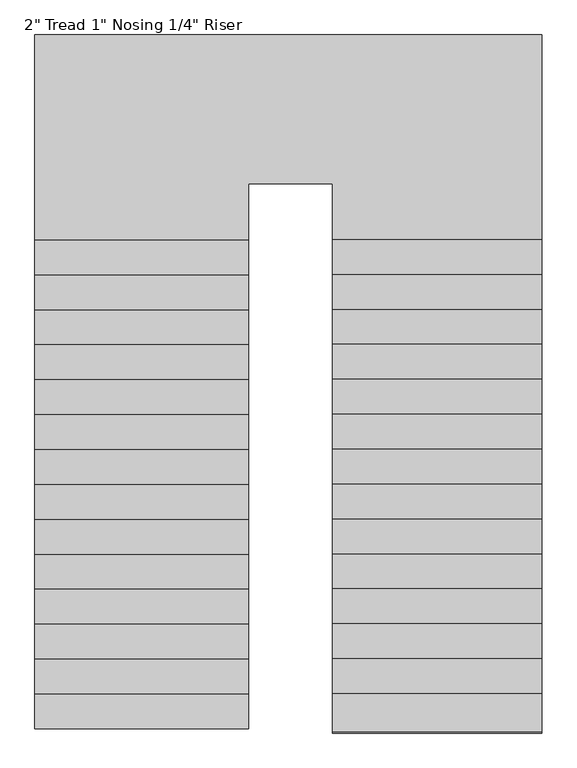
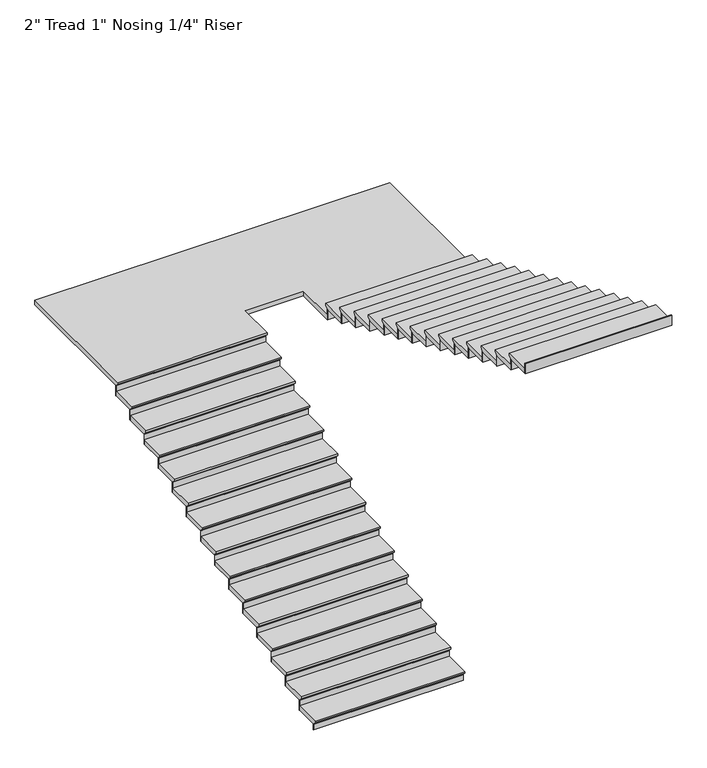
"""IFC4 building model written with IfcOpenShell, lengths in millimetres: stair flight geometry."""

from ifc_helpers import new_model, si_unit, origin, place, context, project, spatial, faceted_brep, source, transform, mapped, element, save


def stair_flight_b71c2a3e(model_context):
    return source(origin(), model_context, "Body", "Brep", [
        faceted_brep([(-5999.9290366, -6973.0610642, -212.09), (-5999.9290366, -6973.0610642, -193.04), (-7554.4415084, -6973.0610642, -193.04), (-7554.4415084, -6973.0610642, -212.09), (-5999.9290366, -6947.6610642, -237.49), (-7554.4415084, -6947.6610642, -237.49), (-5999.9290366, -6693.6610642, -193.04), (-7554.4415084, -6693.6610642, -193.04), (-7554.4415084, -6947.6610642, -243.84), (-7554.4415084, -6693.6610642, -243.84), (-5999.9290366, -6693.6610642, -243.84), (-5999.9290366, -6947.6610642, -243.84)], [[[0, 1, 2, 3]], [[4, 0, 3, 5]], [[2, 1, 6, 7]], [[8, 9, 10, 11]], [[2, 7, 9, 8, 5, 3]], [[8, 11, 4, 5]], [[6, 1, 0, 4, 11, 10]], [[7, 6, 10, 9]]]),
        faceted_brep([(-5999.9290366, -6947.6610642, -243.84), (-5999.9290366, -6947.6610642, -304.8), (-5999.9290366, -6941.3110642, -304.8), (-5999.9290366, -6941.3110642, -243.84), (-7554.4415084, -6947.6610642, -243.84), (-7554.4415084, -6941.3110642, -243.84), (-7554.4415084, -6941.3110642, -304.8), (-7554.4415084, -6947.6610642, -304.8)], [[[0, 1, 2, 3]], [[4, 5, 6, 7]], [[1, 0, 4, 7]], [[2, 1, 7, 6]], [[3, 2, 6, 5]], [[0, 3, 5, 4]]]),
        faceted_brep([(-5999.9290366, -6693.6610642, -132.08), (-5999.9290366, -6693.6610642, -243.84), (-5999.9290366, -6687.3110642, -243.84), (-5999.9290366, -6687.3110642, -132.08), (-7554.4415084, -6693.6610642, -132.08), (-7554.4415084, -6687.3110642, -132.08), (-7554.4415084, -6687.3110642, -243.84), (-7554.4415084, -6693.6610642, -243.84)], [[[0, 1, 2, 3]], [[4, 5, 6, 7]], [[1, 0, 4, 7]], [[2, 1, 7, 6]], [[3, 2, 6, 5]], [[0, 3, 5, 4]]]),
        faceted_brep([(-7554.4415084, -6719.0610642, -81.28), (-5999.9290366, -6719.0610642, -81.28), (-5999.9290366, -6439.6610642, -81.28), (-7554.4415084, -6439.6610642, -81.28), (-7554.4415084, -6693.6610642, -132.08), (-7554.4415084, -6439.6610642, -132.08), (-5999.9290366, -6439.6610642, -132.08), (-5999.9290366, -6693.6610642, -132.08), (-7554.4415084, -6693.6610642, -125.73), (-7554.4415084, -6719.0610642, -100.33), (-5999.9290366, -6693.6610642, -125.73), (-5999.9290366, -6719.0610642, -100.33)], [[[0, 1, 2, 3]], [[4, 5, 6, 7]], [[0, 3, 5, 4, 8, 9]], [[4, 7, 10, 8]], [[2, 1, 11, 10, 7, 6]], [[3, 2, 6, 5]], [[11, 1, 0, 9]], [[10, 11, 9, 8]]]),
        faceted_brep([(-5999.9290366, -6439.6610642, -20.32), (-5999.9290366, -6439.6610642, -132.08), (-5999.9290366, -6433.3110642, -132.08), (-5999.9290366, -6433.3110642, -20.32), (-7554.4415084, -6439.6610642, -20.32), (-7554.4415084, -6433.3110642, -20.32), (-7554.4415084, -6433.3110642, -132.08), (-7554.4415084, -6439.6610642, -132.08)], [[[0, 1, 2, 3]], [[4, 5, 6, 7]], [[1, 0, 4, 7]], [[2, 1, 7, 6]], [[3, 2, 6, 5]], [[0, 3, 5, 4]]]),
        faceted_brep([(-7554.4415084, -6465.0610642, 30.48), (-5999.9290366, -6465.0610642, 30.48), (-5999.9290366, -6185.6610642, 30.48), (-7554.4415084, -6185.6610642, 30.48), (-7554.4415084, -6439.6610642, -20.32), (-7554.4415084, -6185.6610642, -20.32), (-5999.9290366, -6185.6610642, -20.32), (-5999.9290366, -6439.6610642, -20.32), (-7554.4415084, -6439.6610642, -13.97), (-7554.4415084, -6465.0610642, 11.43), (-5999.9290366, -6439.6610642, -13.97), (-5999.9290366, -6465.0610642, 11.43)], [[[0, 1, 2, 3]], [[4, 5, 6, 7]], [[0, 3, 5, 4, 8, 9]], [[4, 7, 10, 8]], [[2, 1, 11, 10, 7, 6]], [[3, 2, 6, 5]], [[11, 1, 0, 9]], [[10, 11, 9, 8]]]),
        faceted_brep([(-5999.9290366, -6185.6610642, 91.44), (-5999.9290366, -6185.6610642, -20.32), (-5999.9290366, -6179.3110642, -20.32), (-5999.9290366, -6179.3110642, 91.44), (-7554.4415084, -6185.6610642, 91.44), (-7554.4415084, -6179.3110642, 91.44), (-7554.4415084, -6179.3110642, -20.32), (-7554.4415084, -6185.6610642, -20.32)], [[[0, 1, 2, 3]], [[4, 5, 6, 7]], [[1, 0, 4, 7]], [[2, 1, 7, 6]], [[3, 2, 6, 5]], [[0, 3, 5, 4]]]),
        faceted_brep([(-7554.4415084, -6211.0610642, 142.24), (-5999.9290366, -6211.0610642, 142.24), (-5999.9290366, -5931.6610642, 142.24), (-7554.4415084, -5931.6610642, 142.24), (-7554.4415084, -6185.6610642, 91.44), (-7554.4415084, -5931.6610642, 91.44), (-5999.9290366, -5931.6610642, 91.44), (-5999.9290366, -6185.6610642, 91.44), (-7554.4415084, -6185.6610642, 97.79), (-7554.4415084, -6211.0610642, 123.19), (-5999.9290366, -6185.6610642, 97.79), (-5999.9290366, -6211.0610642, 123.19)], [[[0, 1, 2, 3]], [[4, 5, 6, 7]], [[0, 3, 5, 4, 8, 9]], [[4, 7, 10, 8]], [[2, 1, 11, 10, 7, 6]], [[3, 2, 6, 5]], [[11, 1, 0, 9]], [[10, 11, 9, 8]]]),
        faceted_brep([(-5999.9290366, -5931.6610642, 203.2), (-5999.9290366, -5931.6610642, 91.44), (-5999.9290366, -5925.3110642, 91.44), (-5999.9290366, -5925.3110642, 203.2), (-7554.4415084, -5931.6610642, 203.2), (-7554.4415084, -5925.3110642, 203.2), (-7554.4415084, -5925.3110642, 91.44), (-7554.4415084, -5931.6610642, 91.44)], [[[0, 1, 2, 3]], [[4, 5, 6, 7]], [[1, 0, 4, 7]], [[2, 1, 7, 6]], [[3, 2, 6, 5]], [[0, 3, 5, 4]]]),
        faceted_brep([(-7554.4415084, -5957.0610642, 254.0), (-5999.9290366, -5957.0610642, 254.0), (-5999.9290366, -5677.6610642, 254.0), (-7554.4415084, -5677.6610642, 254.0), (-7554.4415084, -5931.6610642, 203.2), (-7554.4415084, -5677.6610642, 203.2), (-5999.9290366, -5677.6610642, 203.2), (-5999.9290366, -5931.6610642, 203.2), (-7554.4415084, -5931.6610642, 209.55), (-7554.4415084, -5957.0610642, 234.95), (-5999.9290366, -5931.6610642, 209.55), (-5999.9290366, -5957.0610642, 234.95)], [[[0, 1, 2, 3]], [[4, 5, 6, 7]], [[0, 3, 5, 4, 8, 9]], [[4, 7, 10, 8]], [[2, 1, 11, 10, 7, 6]], [[3, 2, 6, 5]], [[11, 1, 0, 9]], [[10, 11, 9, 8]]]),
        faceted_brep([(-5999.9290366, -5677.6610642, 314.96), (-5999.9290366, -5677.6610642, 203.2), (-5999.9290366, -5671.3110642, 203.2), (-5999.9290366, -5671.3110642, 314.96), (-7554.4415084, -5677.6610642, 314.96), (-7554.4415084, -5671.3110642, 314.96), (-7554.4415084, -5671.3110642, 203.2), (-7554.4415084, -5677.6610642, 203.2)], [[[0, 1, 2, 3]], [[4, 5, 6, 7]], [[1, 0, 4, 7]], [[2, 1, 7, 6]], [[3, 2, 6, 5]], [[0, 3, 5, 4]]]),
        faceted_brep([(-7554.4415084, -5703.0610642, 365.76), (-5999.9290366, -5703.0610642, 365.76), (-5999.9290366, -5423.6610642, 365.76), (-7554.4415084, -5423.6610642, 365.76), (-7554.4415084, -5677.6610642, 314.96), (-7554.4415084, -5423.6610642, 314.96), (-5999.9290366, -5423.6610642, 314.96), (-5999.9290366, -5677.6610642, 314.96), (-7554.4415084, -5677.6610642, 321.31), (-7554.4415084, -5703.0610642, 346.71), (-5999.9290366, -5677.6610642, 321.31), (-5999.9290366, -5703.0610642, 346.71)], [[[0, 1, 2, 3]], [[4, 5, 6, 7]], [[0, 3, 5, 4, 8, 9]], [[4, 7, 10, 8]], [[2, 1, 11, 10, 7, 6]], [[3, 2, 6, 5]], [[11, 1, 0, 9]], [[10, 11, 9, 8]]]),
        faceted_brep([(-5999.9290366, -5423.6610642, 426.72), (-5999.9290366, -5423.6610642, 314.96), (-5999.9290366, -5417.3110642, 314.96), (-5999.9290366, -5417.3110642, 426.72), (-7554.4415084, -5423.6610642, 426.72), (-7554.4415084, -5417.3110642, 426.72), (-7554.4415084, -5417.3110642, 314.96), (-7554.4415084, -5423.6610642, 314.96)], [[[0, 1, 2, 3]], [[4, 5, 6, 7]], [[1, 0, 4, 7]], [[2, 1, 7, 6]], [[3, 2, 6, 5]], [[0, 3, 5, 4]]]),
        faceted_brep([(-7554.4415084, -5449.0610642, 477.52), (-5999.9290366, -5449.0610642, 477.52), (-5999.9290366, -5169.6610642, 477.52), (-7554.4415084, -5169.6610642, 477.52), (-7554.4415084, -5423.6610642, 426.72), (-7554.4415084, -5169.6610642, 426.72), (-5999.9290366, -5169.6610642, 426.72), (-5999.9290366, -5423.6610642, 426.72), (-7554.4415084, -5423.6610642, 433.07), (-7554.4415084, -5449.0610642, 458.47), (-5999.9290366, -5423.6610642, 433.07), (-5999.9290366, -5449.0610642, 458.47)], [[[0, 1, 2, 3]], [[4, 5, 6, 7]], [[0, 3, 5, 4, 8, 9]], [[4, 7, 10, 8]], [[2, 1, 11, 10, 7, 6]], [[3, 2, 6, 5]], [[11, 1, 0, 9]], [[10, 11, 9, 8]]]),
        faceted_brep([(-5999.9290366, -5169.6610642, 538.48), (-5999.9290366, -5169.6610642, 426.72), (-5999.9290366, -5163.3110642, 426.72), (-5999.9290366, -5163.3110642, 538.48), (-7554.4415084, -5169.6610642, 538.48), (-7554.4415084, -5163.3110642, 538.48), (-7554.4415084, -5163.3110642, 426.72), (-7554.4415084, -5169.6610642, 426.72)], [[[0, 1, 2, 3]], [[4, 5, 6, 7]], [[1, 0, 4, 7]], [[2, 1, 7, 6]], [[3, 2, 6, 5]], [[0, 3, 5, 4]]]),
        faceted_brep([(-7554.4415084, -5195.0610642, 589.28), (-5999.9290366, -5195.0610642, 589.28), (-5999.9290366, -4915.6610642, 589.28), (-7554.4415084, -4915.6610642, 589.28), (-7554.4415084, -5169.6610642, 538.48), (-7554.4415084, -4915.6610642, 538.48), (-5999.9290366, -4915.6610642, 538.48), (-5999.9290366, -5169.6610642, 538.48), (-7554.4415084, -5169.6610642, 544.83), (-7554.4415084, -5195.0610642, 570.23), (-5999.9290366, -5169.6610642, 544.83), (-5999.9290366, -5195.0610642, 570.23)], [[[0, 1, 2, 3]], [[4, 5, 6, 7]], [[0, 3, 5, 4, 8, 9]], [[4, 7, 10, 8]], [[2, 1, 11, 10, 7, 6]], [[3, 2, 6, 5]], [[11, 1, 0, 9]], [[10, 11, 9, 8]]]),
        faceted_brep([(-5999.9290366, -4915.6610642, 650.24), (-5999.9290366, -4915.6610642, 538.48), (-5999.9290366, -4909.3110642, 538.48), (-5999.9290366, -4909.3110642, 650.24), (-7554.4415084, -4915.6610642, 650.24), (-7554.4415084, -4909.3110642, 650.24), (-7554.4415084, -4909.3110642, 538.48), (-7554.4415084, -4915.6610642, 538.48)], [[[0, 1, 2, 3]], [[4, 5, 6, 7]], [[1, 0, 4, 7]], [[2, 1, 7, 6]], [[3, 2, 6, 5]], [[0, 3, 5, 4]]]),
        faceted_brep([(-7554.4415084, -4941.0610642, 701.04), (-5999.9290366, -4941.0610642, 701.04), (-5999.9290366, -4661.6610642, 701.04), (-7554.4415084, -4661.6610642, 701.04), (-7554.4415084, -4915.6610642, 650.24), (-7554.4415084, -4661.6610642, 650.24), (-5999.9290366, -4661.6610642, 650.24), (-5999.9290366, -4915.6610642, 650.24), (-7554.4415084, -4915.6610642, 656.59), (-7554.4415084, -4941.0610642, 681.99), (-5999.9290366, -4915.6610642, 656.59), (-5999.9290366, -4941.0610642, 681.99)], [[[0, 1, 2, 3]], [[4, 5, 6, 7]], [[0, 3, 5, 4, 8, 9]], [[4, 7, 10, 8]], [[2, 1, 11, 10, 7, 6]], [[3, 2, 6, 5]], [[11, 1, 0, 9]], [[10, 11, 9, 8]]]),
        faceted_brep([(-5999.9290366, -4661.6610642, 762.0), (-5999.9290366, -4661.6610642, 650.24), (-5999.9290366, -4655.3110642, 650.24), (-5999.9290366, -4655.3110642, 762.0), (-7554.4415084, -4661.6610642, 762.0), (-7554.4415084, -4655.3110642, 762.0), (-7554.4415084, -4655.3110642, 650.24), (-7554.4415084, -4661.6610642, 650.24)], [[[0, 1, 2, 3]], [[4, 5, 6, 7]], [[1, 0, 4, 7]], [[2, 1, 7, 6]], [[3, 2, 6, 5]], [[0, 3, 5, 4]]]),
        faceted_brep([(-7554.4415084, -4687.0610642, 812.8), (-5999.9290366, -4687.0610642, 812.8), (-5999.9290366, -4407.6610642, 812.8), (-7554.4415084, -4407.6610642, 812.8), (-7554.4415084, -4661.6610642, 762.0), (-7554.4415084, -4407.6610642, 762.0), (-5999.9290366, -4407.6610642, 762.0), (-5999.9290366, -4661.6610642, 762.0), (-7554.4415084, -4661.6610642, 768.35), (-7554.4415084, -4687.0610642, 793.75), (-5999.9290366, -4661.6610642, 768.35), (-5999.9290366, -4687.0610642, 793.75)], [[[0, 1, 2, 3]], [[4, 5, 6, 7]], [[0, 3, 5, 4, 8, 9]], [[4, 7, 10, 8]], [[2, 1, 11, 10, 7, 6]], [[3, 2, 6, 5]], [[11, 1, 0, 9]], [[10, 11, 9, 8]]]),
        faceted_brep([(-5999.9290366, -4407.6610642, 873.76), (-5999.9290366, -4407.6610642, 762.0), (-5999.9290366, -4401.3110642, 762.0), (-5999.9290366, -4401.3110642, 873.76), (-7554.4415084, -4407.6610642, 873.76), (-7554.4415084, -4401.3110642, 873.76), (-7554.4415084, -4401.3110642, 762.0), (-7554.4415084, -4407.6610642, 762.0)], [[[0, 1, 2, 3]], [[4, 5, 6, 7]], [[1, 0, 4, 7]], [[2, 1, 7, 6]], [[3, 2, 6, 5]], [[0, 3, 5, 4]]]),
        faceted_brep([(-7554.4415084, -4433.0610642, 924.56), (-5999.9290366, -4433.0610642, 924.56), (-5999.9290366, -4153.6610642, 924.56), (-7554.4415084, -4153.6610642, 924.56), (-7554.4415084, -4407.6610642, 873.76), (-7554.4415084, -4153.6610642, 873.76), (-5999.9290366, -4153.6610642, 873.76), (-5999.9290366, -4407.6610642, 873.76), (-7554.4415084, -4407.6610642, 880.11), (-7554.4415084, -4433.0610642, 905.51), (-5999.9290366, -4407.6610642, 880.11), (-5999.9290366, -4433.0610642, 905.51)], [[[0, 1, 2, 3]], [[4, 5, 6, 7]], [[0, 3, 5, 4, 8, 9]], [[4, 7, 10, 8]], [[2, 1, 11, 10, 7, 6]], [[3, 2, 6, 5]], [[11, 1, 0, 9]], [[10, 11, 9, 8]]]),
        faceted_brep([(-5999.9290366, -4153.6610642, 985.52), (-5999.9290366, -4153.6610642, 873.76), (-5999.9290366, -4147.3110642, 873.76), (-5999.9290366, -4147.3110642, 985.52), (-7554.4415084, -4153.6610642, 985.52), (-7554.4415084, -4147.3110642, 985.52), (-7554.4415084, -4147.3110642, 873.76), (-7554.4415084, -4153.6610642, 873.76)], [[[0, 1, 2, 3]], [[4, 5, 6, 7]], [[1, 0, 4, 7]], [[2, 1, 7, 6]], [[3, 2, 6, 5]], [[0, 3, 5, 4]]]),
        faceted_brep([(-7554.4415084, -4179.0610642, 1036.32), (-5999.9290366, -4179.0610642, 1036.32), (-5999.9290366, -3899.6610642, 1036.32), (-7554.4415084, -3899.6610642, 1036.32), (-7554.4415084, -4153.6610642, 985.52), (-7554.4415084, -3899.6610642, 985.52), (-5999.9290366, -3899.6610642, 985.52), (-5999.9290366, -4153.6610642, 985.52), (-7554.4415084, -4153.6610642, 991.87), (-7554.4415084, -4179.0610642, 1017.27), (-5999.9290366, -4153.6610642, 991.87), (-5999.9290366, -4179.0610642, 1017.27)], [[[0, 1, 2, 3]], [[4, 5, 6, 7]], [[0, 3, 5, 4, 8, 9]], [[4, 7, 10, 8]], [[2, 1, 11, 10, 7, 6]], [[3, 2, 6, 5]], [[11, 1, 0, 9]], [[10, 11, 9, 8]]]),
        faceted_brep([(-5999.9290366, -3899.6610642, 1097.28), (-5999.9290366, -3899.6610642, 985.52), (-5999.9290366, -3893.3110642, 985.52), (-5999.9290366, -3893.3110642, 1097.28), (-7554.4415084, -3899.6610642, 1097.28), (-7554.4415084, -3893.3110642, 1097.28), (-7554.4415084, -3893.3110642, 985.52), (-7554.4415084, -3899.6610642, 985.52)], [[[0, 1, 2, 3]], [[4, 5, 6, 7]], [[1, 0, 4, 7]], [[2, 1, 7, 6]], [[3, 2, 6, 5]], [[0, 3, 5, 4]]]),
        faceted_brep([(-7554.4415084, -3925.0610642, 1148.08), (-5999.9290366, -3925.0610642, 1148.08), (-5999.9290366, -3645.6610642, 1148.08), (-7554.4415084, -3645.6610642, 1148.08), (-7554.4415084, -3899.6610642, 1097.28), (-7554.4415084, -3645.6610642, 1097.28), (-5999.9290366, -3645.6610642, 1097.28), (-5999.9290366, -3899.6610642, 1097.28), (-7554.4415084, -3899.6610642, 1103.63), (-7554.4415084, -3925.0610642, 1129.03), (-5999.9290366, -3899.6610642, 1103.63), (-5999.9290366, -3925.0610642, 1129.03)], [[[0, 1, 2, 3]], [[4, 5, 6, 7]], [[0, 3, 5, 4, 8, 9]], [[4, 7, 10, 8]], [[2, 1, 11, 10, 7, 6]], [[3, 2, 6, 5]], [[11, 1, 0, 9]], [[10, 11, 9, 8]]]),
        faceted_brep([(-5999.9290366, -3645.6610642, 1209.04), (-5999.9290366, -3645.6610642, 1097.28), (-5999.9290366, -3639.3110642, 1097.28), (-5999.9290366, -3639.3110642, 1209.04), (-7554.4415084, -3645.6610642, 1209.04), (-7554.4415084, -3639.3110642, 1209.04), (-7554.4415084, -3639.3110642, 1097.28), (-7554.4415084, -3645.6610642, 1097.28)], [[[0, 1, 2, 3]], [[4, 5, 6, 7]], [[1, 0, 4, 7]], [[2, 1, 7, 6]], [[3, 2, 6, 5]], [[0, 3, 5, 4]]]),
        faceted_brep([(-7554.4415084, -3671.0610642, 1259.84), (-5999.9290366, -3671.0610642, 1259.84), (-5999.9290366, -3391.6610642, 1259.84), (-7554.4415084, -3391.6610642, 1259.84), (-7554.4415084, -3645.6610642, 1209.04), (-7554.4415084, -3391.6610642, 1209.04), (-5999.9290366, -3391.6610642, 1209.04), (-5999.9290366, -3645.6610642, 1209.04), (-7554.4415084, -3645.6610642, 1215.39), (-7554.4415084, -3671.0610642, 1240.79), (-5999.9290366, -3645.6610642, 1215.39), (-5999.9290366, -3671.0610642, 1240.79)], [[[0, 1, 2, 3]], [[4, 5, 6, 7]], [[0, 3, 5, 4, 8, 9]], [[4, 7, 10, 8]], [[2, 1, 11, 10, 7, 6]], [[3, 2, 6, 5]], [[11, 1, 0, 9]], [[10, 11, 9, 8]]]),
        faceted_brep([(-5999.9290366, -3391.6610642, 1320.8), (-5999.9290366, -3391.6610642, 1209.04), (-5999.9290366, -3385.3110642, 1209.04), (-5999.9290366, -3385.3110642, 1320.8), (-7554.4415084, -3391.6610642, 1320.8), (-7554.4415084, -3385.3110642, 1320.8), (-7554.4415084, -3385.3110642, 1209.04), (-7554.4415084, -3391.6610642, 1209.04)], [[[0, 1, 2, 3]], [[4, 5, 6, 7]], [[1, 0, 4, 7]], [[2, 1, 7, 6]], [[3, 2, 6, 5]], [[0, 3, 5, 4]]]),
        faceted_brep([(-3866.3290366, -3442.4610642, 1371.6), (-3866.3290366, -1928.4217109, 1371.6), (-7554.4415084, -1928.4217109, 1371.6), (-7554.4415084, -3417.0610642, 1371.6), (-5999.9290366, -3417.0610642, 1371.6), (-5999.9290366, -3010.6610642, 1371.6), (-5390.3290366, -3010.6610642, 1371.6), (-5390.3290366, -3442.4610642, 1371.6), (-3866.3290366, -1928.4217109, 1320.8), (-3866.3290366, -3442.4610642, 1320.8), (-5390.3290366, -3442.4610642, 1320.8), (-5390.3290366, -3010.6610642, 1320.8), (-5999.9290366, -3010.6610642, 1320.8), (-5999.9290366, -3391.6610642, 1320.8), (-7554.4415084, -3391.6610642, 1320.8), (-7554.4415084, -1928.4217109, 1320.8), (-7554.4415084, -3391.6610642, 1327.15), (-7554.4415084, -3417.0610642, 1352.55), (-5999.9290366, -3391.6610642, 1327.15), (-5999.9290366, -3417.0610642, 1352.55)], [[[0, 1, 2, 3, 4, 5, 6, 7]], [[8, 9, 10, 11, 12, 13, 14, 15]], [[1, 0, 9, 8]], [[2, 1, 8, 15]], [[3, 2, 15, 14, 16, 17]], [[14, 13, 18, 16]], [[5, 4, 19, 18, 13, 12]], [[6, 5, 12, 11]], [[7, 6, 11, 10]], [[0, 7, 10, 9]], [[19, 4, 3, 17]], [[18, 19, 17, 16]]]),
        faceted_brep([(-5390.3290366, -3442.4610642, 1432.56), (-5390.3290366, -3442.4610642, 1320.8), (-5390.3290366, -3448.8110642, 1320.8), (-5390.3290366, -3448.8110642, 1432.56), (-3866.3290366, -3442.4610642, 1432.56), (-3866.3290366, -3448.8110642, 1432.56), (-3866.3290366, -3448.8110642, 1320.8), (-3866.3290366, -3442.4610642, 1320.8)], [[[0, 1, 2, 3]], [[4, 5, 6, 7]], [[1, 0, 4, 7]], [[2, 1, 7, 6]], [[3, 2, 6, 5]], [[0, 3, 5, 4]]]),
        faceted_brep([(-3866.3290366, -3417.0610642, 1483.36), (-5390.3290366, -3417.0610642, 1483.36), (-5390.3290366, -3696.4610642, 1483.36), (-3866.3290366, -3696.4610642, 1483.36), (-3866.3290366, -3442.4610642, 1432.56), (-3866.3290366, -3696.4610642, 1432.56), (-5390.3290366, -3696.4610642, 1432.56), (-5390.3290366, -3442.4610642, 1432.56), (-3866.3290366, -3442.4610642, 1438.91), (-3866.3290366, -3417.0610642, 1464.31), (-5390.3290366, -3442.4610642, 1438.91), (-5390.3290366, -3417.0610642, 1464.31)], [[[0, 1, 2, 3]], [[4, 5, 6, 7]], [[0, 3, 5, 4, 8, 9]], [[4, 7, 10, 8]], [[2, 1, 11, 10, 7, 6]], [[3, 2, 6, 5]], [[11, 1, 0, 9]], [[10, 11, 9, 8]]]),
        faceted_brep([(-5390.3290366, -3696.4610642, 1544.32), (-5390.3290366, -3696.4610642, 1432.56), (-5390.3290366, -3702.8110642, 1432.56), (-5390.3290366, -3702.8110642, 1544.32), (-3866.3290366, -3696.4610642, 1544.32), (-3866.3290366, -3702.8110642, 1544.32), (-3866.3290366, -3702.8110642, 1432.56), (-3866.3290366, -3696.4610642, 1432.56)], [[[0, 1, 2, 3]], [[4, 5, 6, 7]], [[1, 0, 4, 7]], [[2, 1, 7, 6]], [[3, 2, 6, 5]], [[0, 3, 5, 4]]]),
        faceted_brep([(-3866.3290366, -3671.0610642, 1595.12), (-5390.3290366, -3671.0610642, 1595.12), (-5390.3290366, -3950.4610642, 1595.12), (-3866.3290366, -3950.4610642, 1595.12), (-3866.3290366, -3696.4610642, 1544.32), (-3866.3290366, -3950.4610642, 1544.32), (-5390.3290366, -3950.4610642, 1544.32), (-5390.3290366, -3696.4610642, 1544.32), (-3866.3290366, -3696.4610642, 1550.67), (-3866.3290366, -3671.0610642, 1576.07), (-5390.3290366, -3696.4610642, 1550.67), (-5390.3290366, -3671.0610642, 1576.07)], [[[0, 1, 2, 3]], [[4, 5, 6, 7]], [[0, 3, 5, 4, 8, 9]], [[4, 7, 10, 8]], [[2, 1, 11, 10, 7, 6]], [[3, 2, 6, 5]], [[11, 1, 0, 9]], [[10, 11, 9, 8]]]),
        faceted_brep([(-5390.3290366, -3950.4610642, 1656.08), (-5390.3290366, -3950.4610642, 1544.32), (-5390.3290366, -3956.8110642, 1544.32), (-5390.3290366, -3956.8110642, 1656.08), (-3866.3290366, -3950.4610642, 1656.08), (-3866.3290366, -3956.8110642, 1656.08), (-3866.3290366, -3956.8110642, 1544.32), (-3866.3290366, -3950.4610642, 1544.32)], [[[0, 1, 2, 3]], [[4, 5, 6, 7]], [[1, 0, 4, 7]], [[2, 1, 7, 6]], [[3, 2, 6, 5]], [[0, 3, 5, 4]]]),
        faceted_brep([(-3866.3290366, -3925.0610642, 1706.88), (-5390.3290366, -3925.0610642, 1706.88), (-5390.3290366, -4204.4610642, 1706.88), (-3866.3290366, -4204.4610642, 1706.88), (-3866.3290366, -3950.4610642, 1656.08), (-3866.3290366, -4204.4610642, 1656.08), (-5390.3290366, -4204.4610642, 1656.08), (-5390.3290366, -3950.4610642, 1656.08), (-3866.3290366, -3950.4610642, 1662.43), (-3866.3290366, -3925.0610642, 1687.83), (-5390.3290366, -3950.4610642, 1662.43), (-5390.3290366, -3925.0610642, 1687.83)], [[[0, 1, 2, 3]], [[4, 5, 6, 7]], [[0, 3, 5, 4, 8, 9]], [[4, 7, 10, 8]], [[2, 1, 11, 10, 7, 6]], [[3, 2, 6, 5]], [[11, 1, 0, 9]], [[10, 11, 9, 8]]]),
        faceted_brep([(-5390.3290366, -4204.4610642, 1767.84), (-5390.3290366, -4204.4610642, 1656.08), (-5390.3290366, -4210.8110642, 1656.08), (-5390.3290366, -4210.8110642, 1767.84), (-3866.3290366, -4204.4610642, 1767.84), (-3866.3290366, -4210.8110642, 1767.84), (-3866.3290366, -4210.8110642, 1656.08), (-3866.3290366, -4204.4610642, 1656.08)], [[[0, 1, 2, 3]], [[4, 5, 6, 7]], [[1, 0, 4, 7]], [[2, 1, 7, 6]], [[3, 2, 6, 5]], [[0, 3, 5, 4]]]),
        faceted_brep([(-3866.3290366, -4179.0610642, 1818.64), (-5390.3290366, -4179.0610642, 1818.64), (-5390.3290366, -4458.4610642, 1818.64), (-3866.3290366, -4458.4610642, 1818.64), (-3866.3290366, -4204.4610642, 1767.84), (-3866.3290366, -4458.4610642, 1767.84), (-5390.3290366, -4458.4610642, 1767.84), (-5390.3290366, -4204.4610642, 1767.84), (-3866.3290366, -4204.4610642, 1774.19), (-3866.3290366, -4179.0610642, 1799.59), (-5390.3290366, -4204.4610642, 1774.19), (-5390.3290366, -4179.0610642, 1799.59)], [[[0, 1, 2, 3]], [[4, 5, 6, 7]], [[0, 3, 5, 4, 8, 9]], [[4, 7, 10, 8]], [[2, 1, 11, 10, 7, 6]], [[3, 2, 6, 5]], [[11, 1, 0, 9]], [[10, 11, 9, 8]]]),
        faceted_brep([(-5390.3290366, -4458.4610642, 1879.6), (-5390.3290366, -4458.4610642, 1767.84), (-5390.3290366, -4464.8110642, 1767.84), (-5390.3290366, -4464.8110642, 1879.6), (-3866.3290366, -4458.4610642, 1879.6), (-3866.3290366, -4464.8110642, 1879.6), (-3866.3290366, -4464.8110642, 1767.84), (-3866.3290366, -4458.4610642, 1767.84)], [[[0, 1, 2, 3]], [[4, 5, 6, 7]], [[1, 0, 4, 7]], [[2, 1, 7, 6]], [[3, 2, 6, 5]], [[0, 3, 5, 4]]]),
        faceted_brep([(-3866.3290366, -4433.0610642, 1930.4), (-5390.3290366, -4433.0610642, 1930.4), (-5390.3290366, -4712.4610642, 1930.4), (-3866.3290366, -4712.4610642, 1930.4), (-3866.3290366, -4458.4610642, 1879.6), (-3866.3290366, -4712.4610642, 1879.6), (-5390.3290366, -4712.4610642, 1879.6), (-5390.3290366, -4458.4610642, 1879.6), (-3866.3290366, -4458.4610642, 1885.95), (-3866.3290366, -4433.0610642, 1911.35), (-5390.3290366, -4458.4610642, 1885.95), (-5390.3290366, -4433.0610642, 1911.35)], [[[0, 1, 2, 3]], [[4, 5, 6, 7]], [[0, 3, 5, 4, 8, 9]], [[4, 7, 10, 8]], [[2, 1, 11, 10, 7, 6]], [[3, 2, 6, 5]], [[11, 1, 0, 9]], [[10, 11, 9, 8]]]),
        faceted_brep([(-5390.3290366, -4712.4610642, 1991.36), (-5390.3290366, -4712.4610642, 1879.6), (-5390.3290366, -4718.8110642, 1879.6), (-5390.3290366, -4718.8110642, 1991.36), (-3866.3290366, -4712.4610642, 1991.36), (-3866.3290366, -4718.8110642, 1991.36), (-3866.3290366, -4718.8110642, 1879.6), (-3866.3290366, -4712.4610642, 1879.6)], [[[0, 1, 2, 3]], [[4, 5, 6, 7]], [[1, 0, 4, 7]], [[2, 1, 7, 6]], [[3, 2, 6, 5]], [[0, 3, 5, 4]]]),
        faceted_brep([(-3866.3290366, -4687.0610642, 2042.16), (-5390.3290366, -4687.0610642, 2042.16), (-5390.3290366, -4966.4610642, 2042.16), (-3866.3290366, -4966.4610642, 2042.16), (-3866.3290366, -4712.4610642, 1991.36), (-3866.3290366, -4966.4610642, 1991.36), (-5390.3290366, -4966.4610642, 1991.36), (-5390.3290366, -4712.4610642, 1991.36), (-3866.3290366, -4712.4610642, 1997.71), (-3866.3290366, -4687.0610642, 2023.11), (-5390.3290366, -4712.4610642, 1997.71), (-5390.3290366, -4687.0610642, 2023.11)], [[[0, 1, 2, 3]], [[4, 5, 6, 7]], [[0, 3, 5, 4, 8, 9]], [[4, 7, 10, 8]], [[2, 1, 11, 10, 7, 6]], [[3, 2, 6, 5]], [[11, 1, 0, 9]], [[10, 11, 9, 8]]]),
        faceted_brep([(-5390.3290366, -4966.4610642, 2103.12), (-5390.3290366, -4966.4610642, 1991.36), (-5390.3290366, -4972.8110642, 1991.36), (-5390.3290366, -4972.8110642, 2103.12), (-3866.3290366, -4966.4610642, 2103.12), (-3866.3290366, -4972.8110642, 2103.12), (-3866.3290366, -4972.8110642, 1991.36), (-3866.3290366, -4966.4610642, 1991.36)], [[[0, 1, 2, 3]], [[4, 5, 6, 7]], [[1, 0, 4, 7]], [[2, 1, 7, 6]], [[3, 2, 6, 5]], [[0, 3, 5, 4]]]),
        faceted_brep([(-3866.3290366, -4941.0610642, 2153.92), (-5390.3290366, -4941.0610642, 2153.92), (-5390.3290366, -5220.4610642, 2153.92), (-3866.3290366, -5220.4610642, 2153.92), (-3866.3290366, -4966.4610642, 2103.12), (-3866.3290366, -5220.4610642, 2103.12), (-5390.3290366, -5220.4610642, 2103.12), (-5390.3290366, -4966.4610642, 2103.12), (-3866.3290366, -4966.4610642, 2109.47), (-3866.3290366, -4941.0610642, 2134.87), (-5390.3290366, -4966.4610642, 2109.47), (-5390.3290366, -4941.0610642, 2134.87)], [[[0, 1, 2, 3]], [[4, 5, 6, 7]], [[0, 3, 5, 4, 8, 9]], [[4, 7, 10, 8]], [[2, 1, 11, 10, 7, 6]], [[3, 2, 6, 5]], [[11, 1, 0, 9]], [[10, 11, 9, 8]]]),
        faceted_brep([(-5390.3290366, -5220.4610642, 2214.88), (-5390.3290366, -5220.4610642, 2103.12), (-5390.3290366, -5226.8110642, 2103.12), (-5390.3290366, -5226.8110642, 2214.88), (-3866.3290366, -5220.4610642, 2214.88), (-3866.3290366, -5226.8110642, 2214.88), (-3866.3290366, -5226.8110642, 2103.12), (-3866.3290366, -5220.4610642, 2103.12)], [[[0, 1, 2, 3]], [[4, 5, 6, 7]], [[1, 0, 4, 7]], [[2, 1, 7, 6]], [[3, 2, 6, 5]], [[0, 3, 5, 4]]]),
        faceted_brep([(-3866.3290366, -5195.0610642, 2265.68), (-5390.3290366, -5195.0610642, 2265.68), (-5390.3290366, -5474.4610642, 2265.68), (-3866.3290366, -5474.4610642, 2265.68), (-3866.3290366, -5220.4610642, 2214.88), (-3866.3290366, -5474.4610642, 2214.88), (-5390.3290366, -5474.4610642, 2214.88), (-5390.3290366, -5220.4610642, 2214.88), (-3866.3290366, -5220.4610642, 2221.23), (-3866.3290366, -5195.0610642, 2246.63), (-5390.3290366, -5220.4610642, 2221.23), (-5390.3290366, -5195.0610642, 2246.63)], [[[0, 1, 2, 3]], [[4, 5, 6, 7]], [[0, 3, 5, 4, 8, 9]], [[4, 7, 10, 8]], [[2, 1, 11, 10, 7, 6]], [[3, 2, 6, 5]], [[11, 1, 0, 9]], [[10, 11, 9, 8]]]),
        faceted_brep([(-5390.3290366, -5474.4610642, 2326.64), (-5390.3290366, -5474.4610642, 2214.88), (-5390.3290366, -5480.8110642, 2214.88), (-5390.3290366, -5480.8110642, 2326.64), (-3866.3290366, -5474.4610642, 2326.64), (-3866.3290366, -5480.8110642, 2326.64), (-3866.3290366, -5480.8110642, 2214.88), (-3866.3290366, -5474.4610642, 2214.88)], [[[0, 1, 2, 3]], [[4, 5, 6, 7]], [[1, 0, 4, 7]], [[2, 1, 7, 6]], [[3, 2, 6, 5]], [[0, 3, 5, 4]]]),
        faceted_brep([(-3866.3290366, -5449.0610642, 2377.44), (-5390.3290366, -5449.0610642, 2377.44), (-5390.3290366, -5728.4610642, 2377.44), (-3866.3290366, -5728.4610642, 2377.44), (-3866.3290366, -5474.4610642, 2326.64), (-3866.3290366, -5728.4610642, 2326.64), (-5390.3290366, -5728.4610642, 2326.64), (-5390.3290366, -5474.4610642, 2326.64), (-3866.3290366, -5474.4610642, 2332.99), (-3866.3290366, -5449.0610642, 2358.39), (-5390.3290366, -5474.4610642, 2332.99), (-5390.3290366, -5449.0610642, 2358.39)], [[[0, 1, 2, 3]], [[4, 5, 6, 7]], [[0, 3, 5, 4, 8, 9]], [[4, 7, 10, 8]], [[2, 1, 11, 10, 7, 6]], [[3, 2, 6, 5]], [[11, 1, 0, 9]], [[10, 11, 9, 8]]]),
        faceted_brep([(-5390.3290366, -5728.4610642, 2438.4), (-5390.3290366, -5728.4610642, 2326.64), (-5390.3290366, -5734.8110642, 2326.64), (-5390.3290366, -5734.8110642, 2438.4), (-3866.3290366, -5728.4610642, 2438.4), (-3866.3290366, -5734.8110642, 2438.4), (-3866.3290366, -5734.8110642, 2326.64), (-3866.3290366, -5728.4610642, 2326.64)], [[[0, 1, 2, 3]], [[4, 5, 6, 7]], [[1, 0, 4, 7]], [[2, 1, 7, 6]], [[3, 2, 6, 5]], [[0, 3, 5, 4]]]),
        faceted_brep([(-3866.3290366, -5703.0610642, 2489.2), (-5390.3290366, -5703.0610642, 2489.2), (-5390.3290366, -5982.4610642, 2489.2), (-3866.3290366, -5982.4610642, 2489.2), (-3866.3290366, -5728.4610642, 2438.4), (-3866.3290366, -5982.4610642, 2438.4), (-5390.3290366, -5982.4610642, 2438.4), (-5390.3290366, -5728.4610642, 2438.4), (-3866.3290366, -5728.4610642, 2444.75), (-3866.3290366, -5703.0610642, 2470.15), (-5390.3290366, -5728.4610642, 2444.75), (-5390.3290366, -5703.0610642, 2470.15)], [[[0, 1, 2, 3]], [[4, 5, 6, 7]], [[0, 3, 5, 4, 8, 9]], [[4, 7, 10, 8]], [[2, 1, 11, 10, 7, 6]], [[3, 2, 6, 5]], [[11, 1, 0, 9]], [[10, 11, 9, 8]]]),
        faceted_brep([(-5390.3290366, -5982.4610642, 2550.16), (-5390.3290366, -5982.4610642, 2438.4), (-5390.3290366, -5988.8110642, 2438.4), (-5390.3290366, -5988.8110642, 2550.16), (-3866.3290366, -5982.4610642, 2550.16), (-3866.3290366, -5988.8110642, 2550.16), (-3866.3290366, -5988.8110642, 2438.4), (-3866.3290366, -5982.4610642, 2438.4)], [[[0, 1, 2, 3]], [[4, 5, 6, 7]], [[1, 0, 4, 7]], [[2, 1, 7, 6]], [[3, 2, 6, 5]], [[0, 3, 5, 4]]]),
        faceted_brep([(-3866.3290366, -5957.0610642, 2600.96), (-5390.3290366, -5957.0610642, 2600.96), (-5390.3290366, -6236.4610642, 2600.96), (-3866.3290366, -6236.4610642, 2600.96), (-3866.3290366, -5982.4610642, 2550.16), (-3866.3290366, -6236.4610642, 2550.16), (-5390.3290366, -6236.4610642, 2550.16), (-5390.3290366, -5982.4610642, 2550.16), (-3866.3290366, -5982.4610642, 2556.51), (-3866.3290366, -5957.0610642, 2581.91), (-5390.3290366, -5982.4610642, 2556.51), (-5390.3290366, -5957.0610642, 2581.91)], [[[0, 1, 2, 3]], [[4, 5, 6, 7]], [[0, 3, 5, 4, 8, 9]], [[4, 7, 10, 8]], [[2, 1, 11, 10, 7, 6]], [[3, 2, 6, 5]], [[11, 1, 0, 9]], [[10, 11, 9, 8]]]),
        faceted_brep([(-5390.3290366, -6236.4610642, 2661.92), (-5390.3290366, -6236.4610642, 2550.16), (-5390.3290366, -6242.8110642, 2550.16), (-5390.3290366, -6242.8110642, 2661.92), (-3866.3290366, -6236.4610642, 2661.92), (-3866.3290366, -6242.8110642, 2661.92), (-3866.3290366, -6242.8110642, 2550.16), (-3866.3290366, -6236.4610642, 2550.16)], [[[0, 1, 2, 3]], [[4, 5, 6, 7]], [[1, 0, 4, 7]], [[2, 1, 7, 6]], [[3, 2, 6, 5]], [[0, 3, 5, 4]]]),
        faceted_brep([(-3866.3290366, -6211.0610642, 2712.72), (-5390.3290366, -6211.0610642, 2712.72), (-5390.3290366, -6490.4610642, 2712.72), (-3866.3290366, -6490.4610642, 2712.72), (-3866.3290366, -6236.4610642, 2661.92), (-3866.3290366, -6490.4610642, 2661.92), (-5390.3290366, -6490.4610642, 2661.92), (-5390.3290366, -6236.4610642, 2661.92), (-3866.3290366, -6236.4610642, 2668.27), (-3866.3290366, -6211.0610642, 2693.67), (-5390.3290366, -6236.4610642, 2668.27), (-5390.3290366, -6211.0610642, 2693.67)], [[[0, 1, 2, 3]], [[4, 5, 6, 7]], [[0, 3, 5, 4, 8, 9]], [[4, 7, 10, 8]], [[2, 1, 11, 10, 7, 6]], [[3, 2, 6, 5]], [[11, 1, 0, 9]], [[10, 11, 9, 8]]]),
        faceted_brep([(-5390.3290366, -6490.4610642, 2773.68), (-5390.3290366, -6490.4610642, 2661.92), (-5390.3290366, -6496.8110642, 2661.92), (-5390.3290366, -6496.8110642, 2773.68), (-3866.3290366, -6490.4610642, 2773.68), (-3866.3290366, -6496.8110642, 2773.68), (-3866.3290366, -6496.8110642, 2661.92), (-3866.3290366, -6490.4610642, 2661.92)], [[[0, 1, 2, 3]], [[4, 5, 6, 7]], [[1, 0, 4, 7]], [[2, 1, 7, 6]], [[3, 2, 6, 5]], [[0, 3, 5, 4]]]),
        faceted_brep([(-3866.3290366, -6465.0610642, 2824.48), (-5390.3290366, -6465.0610642, 2824.48), (-5390.3290366, -6744.4610642, 2824.48), (-3866.3290366, -6744.4610642, 2824.48), (-3866.3290366, -6490.4610642, 2773.68), (-3866.3290366, -6744.4610642, 2773.68), (-5390.3290366, -6744.4610642, 2773.68), (-5390.3290366, -6490.4610642, 2773.68), (-3866.3290366, -6490.4610642, 2780.03), (-3866.3290366, -6465.0610642, 2805.43), (-5390.3290366, -6490.4610642, 2780.03), (-5390.3290366, -6465.0610642, 2805.43)], [[[0, 1, 2, 3]], [[4, 5, 6, 7]], [[0, 3, 5, 4, 8, 9]], [[4, 7, 10, 8]], [[2, 1, 11, 10, 7, 6]], [[3, 2, 6, 5]], [[11, 1, 0, 9]], [[10, 11, 9, 8]]]),
        faceted_brep([(-5390.3290366, -6744.4610642, 2885.44), (-5390.3290366, -6744.4610642, 2773.68), (-5390.3290366, -6750.8110642, 2773.68), (-5390.3290366, -6750.8110642, 2885.44), (-3866.3290366, -6744.4610642, 2885.44), (-3866.3290366, -6750.8110642, 2885.44), (-3866.3290366, -6750.8110642, 2773.68), (-3866.3290366, -6744.4610642, 2773.68)], [[[0, 1, 2, 3]], [[4, 5, 6, 7]], [[1, 0, 4, 7]], [[2, 1, 7, 6]], [[3, 2, 6, 5]], [[0, 3, 5, 4]]]),
        faceted_brep([(-5390.3290366, -6998.4610642, 2997.2), (-5390.3290366, -6998.4610642, 2885.44), (-5390.3290366, -7004.8110642, 2885.44), (-5390.3290366, -7004.8110642, 2997.2), (-3866.3290366, -6998.4610642, 2997.2), (-3866.3290366, -7004.8110642, 2997.2), (-3866.3290366, -7004.8110642, 2885.44), (-3866.3290366, -6998.4610642, 2885.44)], [[[0, 1, 2, 3]], [[4, 5, 6, 7]], [[1, 0, 4, 7]], [[2, 1, 7, 6]], [[3, 2, 6, 5]], [[0, 3, 5, 4]]]),
        faceted_brep([(-3866.3290366, -6719.0610642, 2936.24), (-5390.3290366, -6719.0610642, 2936.24), (-5390.3290366, -6998.4610642, 2936.24), (-3866.3290366, -6998.4610642, 2936.24), (-3866.3290366, -6744.4610642, 2885.44), (-3866.3290366, -6998.4610642, 2885.44), (-5390.3290366, -6998.4610642, 2885.44), (-5390.3290366, -6744.4610642, 2885.44), (-3866.3290366, -6744.4610642, 2891.79), (-3866.3290366, -6719.0610642, 2917.19), (-5390.3290366, -6744.4610642, 2891.79), (-5390.3290366, -6719.0610642, 2917.19)], [[[0, 1, 2, 3]], [[4, 5, 6, 7]], [[0, 3, 5, 4, 8, 9]], [[4, 7, 10, 8]], [[2, 1, 11, 10, 7, 6]], [[3, 2, 6, 5]], [[11, 1, 0, 9]], [[10, 11, 9, 8]]]),
    ])


if __name__ == "__main__":
    model = new_model("IFC4")
    model_context = context("Model", 3, world=origin())
    ifc_project = project(units=[si_unit("LENGTHUNIT", "METRE", prefix="MILLI")], contexts=[model_context])
    site = spatial("IfcSite", under=ifc_project)
    building = spatial("IfcBuilding", under=site)
    placement = place(None, origin())
    stair_flight_shape = stair_flight_b71c2a3e(model_context)
    element("IfcStairFlight", 1, ObjectType="2\" Tread 1\" Nosing 1/4\" Riser", at=placement, inside=building, context=model_context, shape_type="MappedRepresentation", body=[
        mapped(stair_flight_shape, transform((0.0, 0.0, 0.0), x_axis=(1.0, 0.0, 0.0), y_axis=(0.0, 1.0, 0.0), z_axis=(0.0, 0.0, 1.0))),
    ])
    save(model, "model.ifc")
